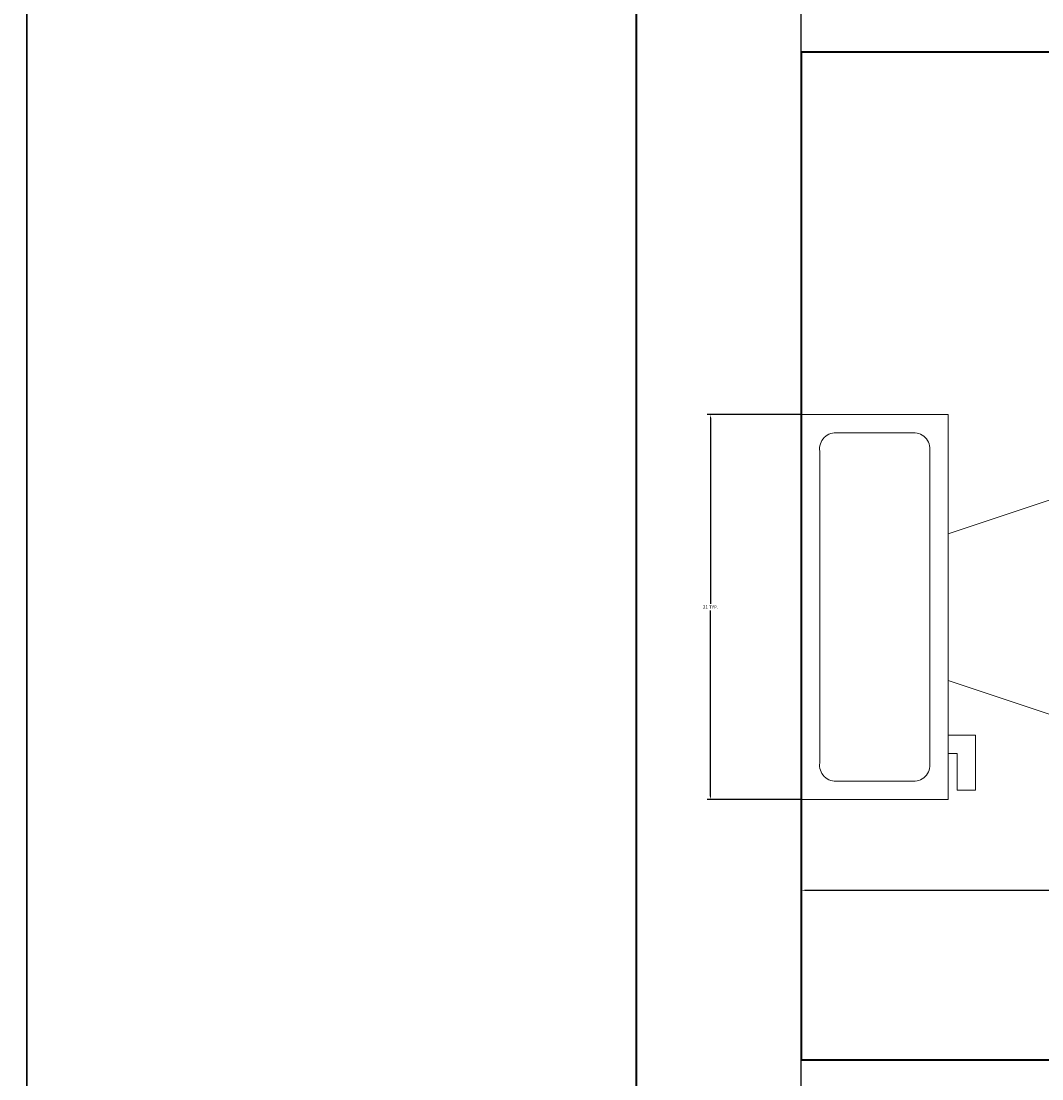
# Model space of a CAD drawing. Units: inches. Extents: x 4159 to 4826, y 299 to 1026.
# Tile 10 of 37: x 4159 to 4214, y 538 to 596. Entities that reach past the tile are written whole.
import ezdxf

# ---------------------------------------------------------------- set-up
doc = ezdxf.new("R2010")
doc.units = ezdxf.units.IN
for name, color, linetype, lineweight in [('A-ANNO-DIMS', 2, 'Continuous', 18), ('A-FLOR-FIXT', 9, 'Continuous', 18), ('A-WALL', 7, 'Continuous', 35)]:
    doc.layers.add(name, color=color, linetype=linetype, lineweight=lineweight)
doc.styles.get("Standard").update_dxf_attribs({"font": 'arial.ttf'})
doc.dimstyles.get("Standard").update_dxf_attribs({"dimtxt": 0.18, "dimasz": 0.18, "dimexe": 0.18, "dimexo": 0.0625, "dimgap": 0.09, "dimtad": 0, "dimtih": 1, "dimtoh": 1, "dimdec": 4, "dimzin": 0, "dimdsep": 46, "dimtxsty": 'Standard', "dimcen": 0.09, "dimadec": 0, "dimazin": 0, "dimtfac": 1, "dimtdec": 4, "dimtofl": 0, "dimtmove": 0, "dimatfit": 3, "dimfxl": 1, "dimtolj": 1, "dimtzin": 0, "dimarcsym": 0})

# ---------------------------------------------------------------- blocks, each defined once
blk = doc.blocks.new('Toilet - top')
for p, q in [((9.5, -6), (9.5, -2)), ((-8, -8.5), (-8, -8)), ((-7, -8), (-7, -9.5)), ((-4, -8), (-6, -14)), ((4, -8), (6, -14)), ((-10, -8.5), (-8, -8.5)), ((-10, -9.5), (-10, -8.5)), ((-7, -9.5), (-10, -9.5)), ((4, -14), (-4, -14))]:
    blk.add_line(p, q)
blk.add_lwpolyline([(10.5, -8), (10.5, 0), (-10.5, 0), (-10.5, -8)], close=True)
for points in [[(8.5, -1), (-8.5, -1)], [(-9.5, -2), (-9.5, -6)], [(-8.5, -7), (8.5, -7)]]:
    blk.add_lwpolyline(points)
for centre, radius, start, end in [((-8.625, -1.875), 0.884, 81.8699, 188.1301), ((8.625, -1.875), 0.884, 351.8699, 98.1301), ((-8.625, -6.125), 0.884, 171.8699, 278.1301), ((8.625, -6.125), 0.884, 261.8699, 8.1301), ((3.52, -21.58), 12.169, 141.46911, 247.97143), ((4.2, -21.817), 11.329, 136.36773, 238.94682), ((-3.519, -21.58), 12.169, 292.02843, 38.53071), ((-4.2, -21.817), 11.329, 301.05301, 43.63209), ((0, -27.876), 4, 245.73182, 294.26817), ((0, -29), 4, 254.86053, 285.13947)]:
    blk.add_arc(centre, radius, start, end)
blk = doc.blocks.new('*D37')
at = {"layer": 'A-ANNO-DIMS', "color": 0, "lineweight": -2, "transparency": 16777216}
for p, q in [((4201.323, 553.415), (4201.323, 548.34)), ((4234.369, 553.415), (4234.369, 548.34)), ((4201.503, 548.52), (4217.07, 548.52)), ((4234.189, 548.52), (4218.622, 548.52))]:
    blk.add_line(p, q, dxfattribs=at)
at = {"layer": 'A-ANNO-DIMS', "color": 0, "transparency": 16777216}
for points in [[(4201.503, 548.55), (4201.503, 548.49), (4201.323, 548.52)], [(4234.189, 548.55), (4234.189, 548.49), (4234.369, 548.52)]]:
    blk.add_solid(points, dxfattribs=at)
at = {"layer": 'Defpoints', "color": 0, "transparency": 16777216}
for p in [(4201.323, 553.477), (4234.369, 553.477), (4201.323, 548.52)]:
    blk.add_point(p, dxfattribs=at)
at = {"layer": 'A-ANNO-DIMS', "color": 0, "transparency": 16777216, "insert": (4217.846, 548.52), "char_height": 0.18, "attachment_point": 5}
blk.add_mtext('\\A1;WC 33 TYP.', dxfattribs=at)
blk = doc.blocks.new('*D38')
at = {"layer": 'A-ANNO-DIMS', "color": 0, "lineweight": -2, "transparency": 16777216}
for p, q in [((4201.26, 574.477), (4196.186, 574.477)), ((4196.366, 574.297), (4196.366, 564.157)), ((4196.366, 553.657), (4196.366, 563.797)), ((4201.26, 553.477), (4196.186, 553.477))]:
    blk.add_line(p, q, dxfattribs=at)
at = {"layer": 'A-ANNO-DIMS', "color": 0, "transparency": 16777216}
for points in [[(4196.336, 574.297), (4196.396, 574.297), (4196.366, 574.477)], [(4196.336, 553.657), (4196.396, 553.657), (4196.366, 553.477)]]:
    blk.add_solid(points, dxfattribs=at)
at = {"layer": 'Defpoints', "color": 0, "transparency": 16777216}
for p in [(4196.366, 574.477), (4201.323, 574.477), (4201.323, 553.477)]:
    blk.add_point(p, dxfattribs=at)
at = {"layer": 'A-ANNO-DIMS', "color": 0, "transparency": 16777216, "insert": (4196.366, 563.977), "char_height": 0.18, "attachment_point": 5}
blk.add_mtext('\\A1;21 TYP.', dxfattribs=at)
blk = doc.blocks.new('*D44')
at = {"layer": 'A-ANNO-DIMS', "color": 0, "lineweight": -2, "transparency": 16777216}
for p, q in [((4287.263, 963.093), (4158.88, 963.093)), ((4159.06, 962.913), (4159.06, 647.826)), ((4159.06, 332.375), (4159.06, 647.462)), ((4447.248, 332.195), (4158.88, 332.195))]:
    blk.add_line(p, q, dxfattribs=at)
at = {"layer": 'A-ANNO-DIMS', "color": 0, "transparency": 16777216}
for points in [[(4159.03, 962.913), (4159.09, 962.913), (4159.06, 963.093)], [(4159.03, 332.375), (4159.09, 332.375), (4159.06, 332.195)]]:
    blk.add_solid(points, dxfattribs=at)
at = {"layer": 'Defpoints', "color": 0, "transparency": 16777216}
for p in [(4287.326, 963.093), (4159.06, 332.195), (4447.31, 332.195)]:
    blk.add_point(p, dxfattribs=at)
at = {"layer": 'A-ANNO-DIMS', "color": 0, "transparency": 16777216, "insert": (4159.06, 647.644), "char_height": 0.18, "attachment_point": 5}
blk.add_mtext('\\A1;630.9', dxfattribs=at)
blk = doc.blocks.new('*D50')
at = {"layer": 'A-ANNO-DIMS', "color": 0, "lineweight": -2, "transparency": 16777216}
for p, q in [((4192.31, 392.317), (4192.31, 1025.842)), ((4192.49, 1025.662), (4196.661, 1025.662)), ((4201.13, 1025.662), (4196.959, 1025.662)), ((4201.31, 401.317), (4201.31, 1025.842))]:
    blk.add_line(p, q, dxfattribs=at)
at = {"layer": 'A-ANNO-DIMS', "color": 0, "transparency": 16777216}
for points in [[(4192.49, 1025.692), (4192.49, 1025.632), (4192.31, 1025.662)], [(4201.13, 1025.692), (4201.13, 1025.632), (4201.31, 1025.662)]]:
    blk.add_solid(points, dxfattribs=at)
at = {"layer": 'Defpoints', "color": 0, "transparency": 16777216}
for p in [(4201.31, 1025.662), (4201.31, 401.254), (4192.31, 392.254)]:
    blk.add_point(p, dxfattribs=at)
at = {"layer": 'A-ANNO-DIMS', "color": 0, "transparency": 16777216, "insert": (4196.81, 1025.662), "char_height": 0.18, "attachment_point": 5}
blk.add_mtext('\\A1;9', dxfattribs=at)
blk = doc.blocks.new('*D51')
at = {"layer": 'A-ANNO-DIMS', "color": 0, "lineweight": -2, "transparency": 16777216}
for p, q in [((4201.248, 660.254), (4158.88, 660.254)), ((4159.06, 660.074), (4159.06, 526.436)), ((4159.06, 392.434), (4159.06, 526.072)), ((4192.248, 392.254), (4158.88, 392.254))]:
    blk.add_line(p, q, dxfattribs=at)
at = {"layer": 'A-ANNO-DIMS', "color": 0, "transparency": 16777216}
for points in [[(4159.03, 660.074), (4159.09, 660.074), (4159.06, 660.254)], [(4159.03, 392.434), (4159.09, 392.434), (4159.06, 392.254)]]:
    blk.add_solid(points, dxfattribs=at)
at = {"layer": 'Defpoints', "color": 0, "transparency": 16777216}
for p in [(4159.06, 660.254), (4201.31, 660.254), (4192.31, 392.254)]:
    blk.add_point(p, dxfattribs=at)
at = {"layer": 'A-ANNO-DIMS', "color": 0, "transparency": 16777216, "insert": (4159.06, 526.254), "char_height": 0.18, "attachment_point": 5}
blk.add_mtext('\\A1;268', dxfattribs=at)

msp = doc.modelspace()

# ---------------------------------------------------------------- linework, layer by layer
at = {"layer": 'A-WALL'}
for p, q in [((4271.31, 594.254), (4201.31, 594.254)), ((4201.31, 594.254), (4201.31, 539.254)), ((4271.31, 539.254), (4201.31, 539.254))]:
    msp.add_line(p, q, dxfattribs=at)
msp.add_lwpolyline([(4303.31, 903.254), (4192.31, 903.254), (4192.31, 392.254)], dxfattribs=at)

# ---------------------------------------------------------------- block references
at = {"layer": 'A-FLOR-FIXT', "rotation": 90}
msp.add_blockref('Toilet - top', (4201.323, 563.977), dxfattribs=at)

# ---------------------------------------------------------------- dimensions: what is measured, and where the dimension line sits
at = {"layer": 'A-ANNO-DIMS'}
dim = msp.add_linear_dim(base=(4201.31, 1025.662), p1=(4192.31, 392.254), p2=(4201.31, 401.254), dimstyle='Standard', override={"dimdec": 0, "dimlfac": 1, "dimrnd": 0, "dimzin": 0, "dimdsep": 46, "dimlunit": 2}, dxfattribs=at)
dim.commit()
dim.dimension.update_dxf_attribs({"geometry": '*D50', "text_midpoint": (4196.81, 1025.662)})
for base, p1, p2, override, picture, middle in [((4159.06, 332.195), (4287.326, 963.093), (4447.31, 332.195), {"dimdec": 1, "dimlfac": 1, "dimrnd": 0, "dimzin": 0, "dimdsep": 46, "dimlunit": 2}, '*D44', (4159.06, 647.644)), ((4159.06, 660.254), (4192.31, 392.254), (4201.31, 660.254), {"dimdec": 0, "dimlfac": 1, "dimrnd": 0, "dimzin": 0, "dimdsep": 46, "dimlunit": 2}, '*D51', (4159.06, 526.254))]:
    dim = msp.add_linear_dim(base=base, p1=p1, p2=p2, angle=90, dimstyle='Standard', override=override, dxfattribs=at)
    dim.commit()
    dim.dimension.update_dxf_attribs({"geometry": picture, "text_midpoint": middle})
for base, p1, p2, angle, text, picture, middle in [((4196.366, 574.477), (4201.323, 553.477), (4201.323, 574.477), 90, '<> TYP.', '*D38', (4196.366, 563.977)), ((4201.323, 548.52), (4234.369, 553.477), (4201.323, 553.477), 180, 'WC <> TYP.', '*D37', (4217.846, 548.52))]:
    dim = msp.add_linear_dim(base=base, p1=p1, p2=p2, angle=angle, text=text, dimstyle='Standard', override={"dimdec": 0, "dimlfac": 1, "dimrnd": 0, "dimzin": 0, "dimdsep": 46, "dimlunit": 2}, dxfattribs=at)
    dim.commit()
    dim.dimension.update_dxf_attribs({"geometry": picture, "text_midpoint": middle})

doc.saveas('drawing.dxf')
